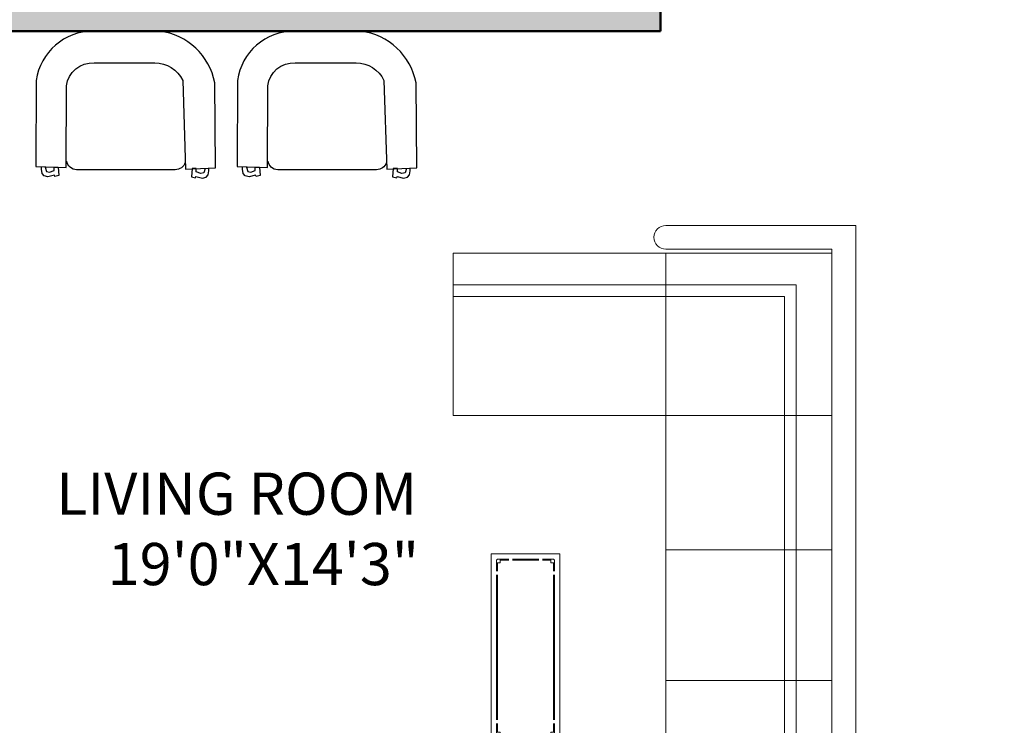
# Model space of a CAD drawing. Units: inches. Extents: x 3008 to 4088, y 1255 to 2137.
# Tile 8 of 30: x 3146 to 3310, y 1670 to 1787. Entities that reach past the tile are written whole.
import ezdxf

# ---------------------------------------------------------------- set-up
doc = ezdxf.new("R2010")
doc.units = ezdxf.units.IN
doc.layers.add('2D', color=7, linetype='Continuous')
for name, color, linetype, lineweight in [('A-AREA-IDEN', 7, 'Continuous', 18), ('A-FURN', 8, 'Continuous', 18), ('A-WALL', 7, 'Continuous', 50), ('A-WALL-PATT', 8, 'Continuous', 13)]:
    doc.layers.add(name, color=color, linetype=linetype, lineweight=lineweight)
doc.styles.get("Standard").update_dxf_attribs({"font": 'arial.ttf'})

# ---------------------------------------------------------------- blocks, each defined once
blk = doc.blocks.new('TABLE-30A')
at = {"color": 0, "linetype": 'ByBlock'}
for p, q in [((0, 0), (0, 0.55)), ((0, 0.55), (1.5, 0.55)), ((0.0508, 0.5077), (0.0423, 0.4992)), ((0.0423, 0.4992), (0.0423, 0.478)), ((0.0423, 0.478), (0.072, 0.478)), ((0.0423, 0.478), (0.0423, 0.4103)), ((0.072, 0.5077), (0.0508, 0.5077)), ((0.0508, 0.478), (0.0508, 0.4103)), ((0.072, 0.478), (0.072, 0.5077)), ((0.072, 0.5077), (0.1397, 0.5077)), ((0.072, 0.4992), (0.1397, 0.4992)), ((1.3307, 0.5077), (0.1693, 0.5077)), ((1.3307, 0.4992), (0.1693, 0.4992)), ((1.428, 0.5077), (1.3603, 0.5077)), ((1.428, 0.4992), (1.3603, 0.4992)), ((1.428, 0.5077), (1.428, 0.478)), ((1.4492, 0.5077), (1.428, 0.5077)), ((1.428, 0.478), (1.4577, 0.478)), ((1.4577, 0.4992), (1.4492, 0.5077)), ((1.4492, 0.478), (1.4492, 0.4103)), ((1.4577, 0.478), (1.4577, 0.4992)), ((1.4577, 0.478), (1.4577, 0.4103)), ((1.5, 0.55), (1.5, 0)), ((0.0423, 0.1693), (0.0423, 0.3807)), ((0.0508, 0.1693), (0.0508, 0.3807)), ((1.4492, 0.3807), (1.4492, 0.1693)), ((1.4577, 0.3807), (1.4577, 0.1693)), ((0.0423, 0.072), (0.0423, 0.1397)), ((0.0508, 0.072), (0.0508, 0.1397)), ((1.4492, 0.072), (1.4492, 0.1397)), ((1.4577, 0.072), (1.4577, 0.1397)), ((1.5, 0), (0, 0)), ((0.0423, 0.072), (0.0423, 0.0508)), ((0.072, 0.072), (0.0423, 0.072)), ((0.0423, 0.0508), (0.0508, 0.0423)), ((0.0508, 0.0423), (0.072, 0.0423)), ((0.072, 0.0423), (0.072, 0.072)), ((0.072, 0.0508), (0.1397, 0.0508)), ((0.072, 0.0423), (0.1397, 0.0423)), ((0.1693, 0.0508), (1.3307, 0.0508)), ((0.1693, 0.0423), (1.3307, 0.0423)), ((1.428, 0.0508), (1.3603, 0.0508)), ((1.428, 0.0423), (1.3603, 0.0423)), ((1.428, 0.072), (1.428, 0.0423)), ((1.4577, 0.072), (1.428, 0.072)), ((1.428, 0.0423), (1.4492, 0.0423)), ((1.4492, 0.0423), (1.4577, 0.0508)), ((1.4577, 0.0508), (1.4577, 0.072))]:
    blk.add_line(p, q, dxfattribs=at)
blk = doc.blocks.new('S 1')
at = {"layer": '2D'}
blk.add_lwpolyline([(4300.17, 1811.07), (4294.36, 1811.27), (4294.5, 1827.76, -0.326306), (4305.18, 1837.77), (4318.07, 1837.77, -0.372891), (4329.09, 1828.23), (4329.16, 1811.54), (4323.28, 1811.34), (4323.21, 1827.16, 0.399039), (4317.87, 1831.63), (4306.12, 1831.63, 0.288471), (4300.71, 1828.23)], format="xyb", close=True, dxfattribs=at)
blk.add_lwpolyline([(4300.24, 1812.34, 0.33845), (4302.18, 1810.94), (4321.28, 1810.94, 0.381322), (4323.15, 1812.61, -0.892406)], format="xyb", dxfattribs=at)
for points in [[(4327.35, 1811.41), (4327.09, 1810.61), (4326.49, 1810.47), (4325.62, 1810.81), (4325.62, 1811.41), (4324.82, 1811.41), (4324.68, 1809.81), (4325.48, 1809.61), (4325.55, 1809.87), (4326.82, 1809.54), (4327.55, 1809.74), (4327.95, 1810.21), (4328.09, 1811.01), (4328.09, 1811.47)], [(4296.37, 1811.14), (4296.63, 1810.34), (4297.23, 1810.21), (4298.1, 1810.54), (4298.1, 1811.14), (4298.9, 1811.14), (4299.04, 1809.54), (4298.24, 1809.34), (4298.17, 1809.61), (4296.9, 1809.27), (4296.17, 1809.47), (4295.77, 1809.94), (4295.63, 1810.74), (4295.63, 1811.21)]]:
    blk.add_lwpolyline(points, dxfattribs=at)
blk = doc.blocks.new('SOFA-L')
for p, q in [((35.53, 102.74), (67.02, 102.74)), ((67.02, 102.74), (67.02, 0.37)), ((0.3, 98.14), (0.3, 71.24)), ((63.09, 98.14), (0.3, 98.14)), ((35.53, 98.8), (63.09, 98.8)), ((35.53, 4.97), (35.53, 98.14)), ((63.09, 98.8), (63.09, 4.97)), ((0.3, 92.9), (57.18, 92.9)), ((57.18, 92.9), (57.18, 4.97)), ((0.3, 90.93), (55.21, 90.93)), ((55.21, 90.93), (55.21, 4.97)), ((63.09, 71.24), (0.3, 71.24)), ((40.78, 71.24), (0.3, 71.24)), ((63.09, 48.93), (35.53, 48.93)), ((63.09, 27.28), (35.53, 27.28)), ((63.09, 9.36), (35.53, 9.36)), ((63.09, 4.97), (35.53, 4.97)), ((67.02, 4.31), (35.53, 4.31)), ((67.02, 0.37), (35.53, 0.37))]:
    blk.add_line(p, q)
for centre in [(35.53, 100.77), (35.53, 2.34)]:
    blk.add_arc(centre, 1.97, 90, 270)

msp = doc.modelspace()

# ---------------------------------------------------------------- hatches: boundary and pattern name
at = {"layer": 'A-WALL-PATT'}
h = msp.add_hatch(color=256, dxfattribs=at)
h.dxf.hatch_style = 1
h.paths.add_polyline_path([(3102.67, 1625.97), (3093.67, 1625.97), (3093.67, 1540.97), (3102.67, 1540.97)])
h.paths.add_polyline_path([(3102.67, 1784.97), (3252.67, 1784.97), (3252.67, 1790.97), (3102.67, 1790.97), (3102.67, 1892.97), (3093.67, 1892.97), (3093.67, 1667.97), (3102.67, 1667.97)])
h.paths.add_polyline_path([(3192.67, 1943.97), (3093.67, 1943.97), (3093.67, 1934.97), (3102.67, 1934.97), (3192.67, 1934.97)])
h.paths.add_polyline_path([(3264.67, 1943.97), (3234.67, 1943.97), (3234.67, 1934.97), (3246.67, 1934.97), (3246.67, 1868.97), (3252.67, 1868.97), (3252.67, 1934.97), (3264.67, 1934.97)])
h.paths.add_polyline_path([(3330.67, 1943.97), (3288.67, 1943.97), (3288.67, 1934.97), (3300.67, 1934.97), (3300.67, 1838.97), (3246.67, 1838.97), (3246.67, 1826.97), (3252.67, 1826.97), (3252.67, 1832.97), (3306.67, 1832.97), (3306.67, 1934.97), (3330.67, 1934.97)])
h.paths.add_polyline_path([(3390.67, 1943.97), (3360.67, 1943.97), (3360.67, 1934.97), (3390.67, 1934.97)])
h.paths.add_polyline_path([(3465.67, 1943.97), (3432.67, 1943.97), (3432.67, 1934.97), (3456.67, 1934.97), (3456.67, 1883.97), (3465.67, 1883.97)])
h.paths.add_polyline_path([(3465.67, 1841.97), (3456.67, 1841.97), (3456.67, 1790.97), (3370.67, 1790.97), (3370.67, 1784.97), (3456.67, 1784.97), (3456.67, 1759.47), (3465.67, 1759.47)])
h.paths.add_polyline_path([(3465.67, 1693.47), (3456.67, 1693.47), (3456.67, 1667.97), (3330.67, 1667.97), (3330.67, 1643.97), (3336.67, 1643.97), (3336.67, 1661.97), (3456.67, 1661.97), (3456.67, 1649.97), (3465.67, 1649.97)])
h.paths.add_polyline_path([(3465.67, 1625.97), (3456.67, 1625.97), (3456.67, 1613.97), (3324.67, 1613.97), (3324.67, 1604.97), (3456.67, 1604.97), (3456.67, 1571.97), (3465.67, 1571.97)])
h.paths.add_polyline_path([(3465.67, 1505.97), (3456.67, 1505.97), (3456.67, 1472.97), (3438.67, 1472.97), (3438.67, 1463.97), (3465.67, 1463.97)])
h.paths.add_polyline_path([(3396.67, 1472.97), (3354.67, 1472.97), (3354.67, 1463.97), (3396.67, 1463.97)])
h.paths.add_polyline_path([(3312.67, 1472.97), (3288.67, 1472.97), (3288.67, 1550.97), (3282.67, 1550.97), (3282.67, 1472.97), (3270.67, 1472.97), (3270.67, 1463.97), (3312.67, 1463.97)])
h.paths.add_polyline_path([(3246.67, 1472.97), (3234.67, 1472.97), (3234.67, 1544.97), (3252.67, 1544.97), (3252.67, 1550.97), (3234.67, 1550.97), (3234.67, 1604.97), (3282.67, 1604.97), (3282.67, 1580.97), (3288.67, 1580.97), (3288.67, 1613.97), (3150.67, 1613.97), (3150.67, 1604.97), (3225.67, 1604.97), (3225.67, 1463.97), (3246.67, 1463.97)])

# ---------------------------------------------------------------- linework, layer by layer
at = {"layer": 'A-WALL'}
for p, q in [((3252.67, 1784.97), (3252.67, 1790.97)), ((3102.67, 1784.97), (3252.67, 1784.97))]:
    msp.add_line(p, q, dxfattribs=at)

# ---------------------------------------------------------------- block references
at = {"layer": 'A-FURN', "xscale": -0.8563117011609614, "yscale": 0.8563117011609614, "zscale": 0.8563117011609614}
for p in [(6856.19, 211.26), (6889.55, 211.26)]:
    msp.add_blockref('S 1', p, dxfattribs=at)
at = {"layer": 'A-FURN'}
msp.add_blockref('SOFA-L', (3218, 1650), dxfattribs=at)
at = {"layer": 'A-FURN', "xscale": 20.70834898381633, "yscale": 20.70834898381633, "zscale": 20.70834898381633, "rotation": 270}
msp.add_blockref('TABLE-30A', (3224.59, 1698.28), dxfattribs=at)

# ---------------------------------------------------------------- texts
at = {"layer": 'A-AREA-IDEN', "insert": (3152.44, 1711.74), "char_height": 7, "attachment_point": 1}
msp.add_mtext_dynamic_manual_height_columns('{\\fTimes New Roman|b0|i0|c0|p18;LIVING ROOM\\P    19\'0"X14\'3"}', width=105.6127, gutter_width=12.5, heights=[0], dxfattribs=at)

doc.saveas('drawing.dxf')
